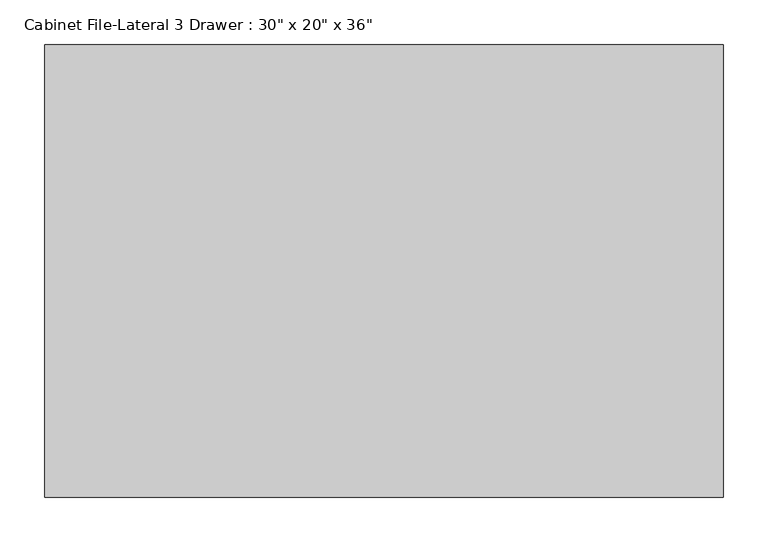
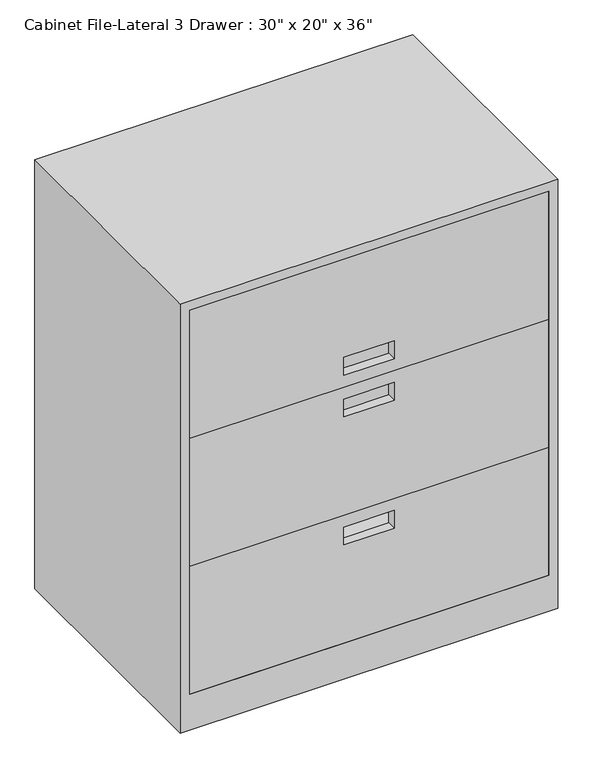
"""IFC4 building model written with IfcOpenShell, lengths in millimetres: furniture geometry."""

from ifc_helpers import new_model, si_unit, frame, origin, place, context, project, spatial, polyline, outline, extrude, faceted_brep, source, transform, mapped, element, save


def furniture_fb07e05e(model_context):
    return source(origin(), model_context, "Body", "SolidModel", [
        faceted_brep([(200.9774861, -680.3183761, 914.4), (-561.0225139, -680.3183761, 914.4), (-561.0225139, -1188.3183761, 914.4), (200.9774861, -1188.3183761, 914.4), (200.9774861, -680.3183761, 0.0), (200.9774861, -1188.3183761, 0.0), (-561.0225139, -1188.3183761, 0.0), (-561.0225139, -680.3183761, 0.0), (181.9274861, -1188.3183761, 76.2), (-541.9725139, -1188.3183761, 76.2), (-541.9725139, -1188.3183761, 895.35), (181.9274861, -1188.3183761, 895.35), (-541.9725139, -699.3683761, 76.2), (181.9274861, -699.3683761, 76.2), (181.9274861, -699.3683761, 895.35), (-541.9725139, -699.3683761, 895.35)], [[[0, 1, 2, 3]], [[4, 5, 6, 7]], [[1, 0, 4, 7]], [[2, 1, 7, 6]], [[3, 2, 6, 5], [8, 9, 10, 11]], [[0, 3, 5, 4]], [[12, 13, 14, 15]], [[13, 12, 9, 8]], [[14, 13, 8, 11]], [[15, 14, 11, 10]], [[12, 15, 10, 9]]]),
        extrude(outline(polyline([(895.35, -541.9725139), (622.2999998, -541.9725139), (622.3, 181.9274861), (895.35, 181.9274861), (895.35, -541.9725139)]), holes=[polyline([(685.8, -230.8225139), (685.8, -129.2225139), (647.7, -129.2225139), (647.7, -230.8225139), (685.8, -230.8225139)])]), frame((0.0, -1188.3183761, 0.0), z_axis=(0.0, 1.0, 0.0), x_axis=(0.0, 0.0, 1.0)), (0.0, 0.0, 1.0), 19.05),
        extrude(outline(polyline([(349.25, -541.9725139), (349.25, 181.9274861), (622.3, 181.9274861), (622.2999998, -541.9725139), (349.25, -541.9725139)]), holes=[polyline([(596.9, -230.8225139), (596.9, -129.2225139), (558.8, -129.2225139), (558.8, -230.8225139), (596.9, -230.8225139)])]), frame((0.0, -1188.3183761, 0.0), z_axis=(0.0, 1.0, 0.0), x_axis=(0.0, 0.0, 1.0)), (0.0, 0.0, 1.0), 19.05),
        extrude(outline(polyline([(76.2, -541.9725139), (76.2, 181.9274861), (349.25, 181.9274861), (349.25, -541.9725139), (76.2, -541.9725139)]), holes=[polyline([(323.85, -230.8225139), (323.85, -129.2225139), (285.75, -129.2225139), (285.75, -230.8225139), (323.85, -230.8225139)])]), frame((0.0, -1188.3183761, 0.0), z_axis=(0.0, 1.0, 0.0), x_axis=(0.0, 0.0, 1.0)), (0.0, 0.0, 1.0), 19.05),
    ])


if __name__ == "__main__":
    model = new_model("IFC4")
    model_context = context("Model", 3, world=origin())
    ifc_project = project(units=[si_unit("LENGTHUNIT", "METRE", prefix="MILLI")], contexts=[model_context])
    site = spatial("IfcSite", under=ifc_project)
    building = spatial("IfcBuilding", under=site)
    placement = place(None, origin())
    furniture_shape = furniture_fb07e05e(model_context)
    element("IfcFurniture", 1, ObjectType="Cabinet File-Lateral 3 Drawer : 30\" x 20\" x 36\"", at=placement, inside=building, context=model_context, shape_type="MappedRepresentation", body=[
        mapped(furniture_shape, transform((0.0, 0.0, 0.0), x_axis=(1.0, 0.0, 0.0), y_axis=(0.0, 1.0, 0.0), z_axis=(0.0, 0.0, 1.0))),
    ])
    save(model, "model.ifc")

# Revit data of these elements
# Type "Cabinet File-Lateral 3 Drawer : 30\" x 20\" x 36\""
#   Assembly Code = "E2020200"
#   Depth = 1' - 8"
#   Height = 3' - 0"
#   Width = 2' - 6"
#   Material = Metal - Steel
#   Default Elevation = 0
# Element 1 (IfcFurniture, "Cabinet File-Lateral 3 Drawer : 30\" x 20\" x 36\"")
#   Materials on its faces: "Metal - Steel"
# Materials
#   "Metal - Steel": colour RGB 209 209 209, transparency 0
